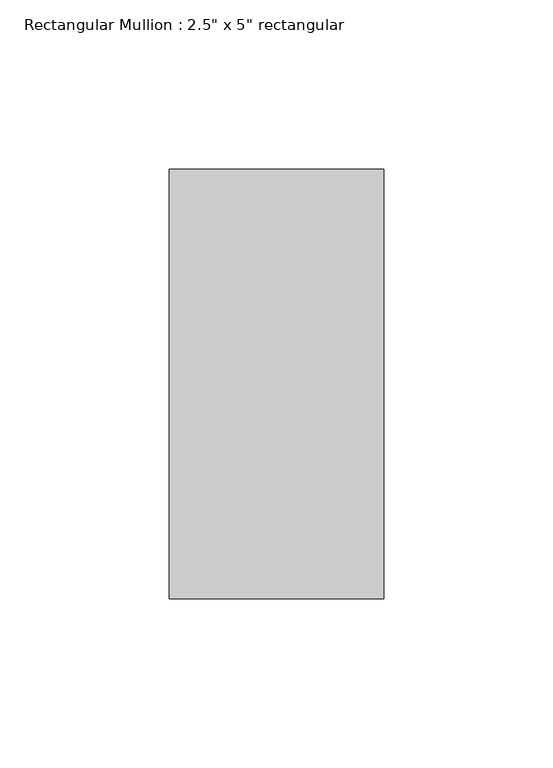
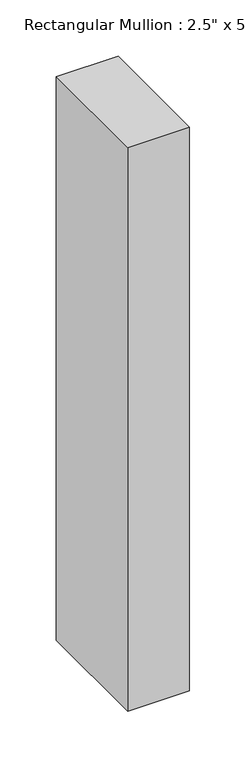
"""IFC4 building model written with IfcOpenShell, lengths in millimetres: member geometry."""

from ifc_helpers import new_model, si_unit, frame, origin, place, context, project, spatial, polyline, outline, extrude, source, transform, mapped, element, save


def member_0fdf3d9d(model_context):
    return source(origin(), model_context, "Body", "SweptSolid", [
        extrude(outline(polyline([(0.0, 63.5), (0.0, -63.5), (-63.5, -63.5), (-63.5, 63.5), (0.0, 63.5)])), frame((0.0, 0.0, -612.775), z_axis=(0.0, 0.0, 1.0), x_axis=(1.0, 0.0, 0.0)), (0.0, 0.0, 1.0), 612.775),
    ])


if __name__ == "__main__":
    model = new_model("IFC4")
    model_context = context("Model", 3, world=origin())
    ifc_project = project(units=[si_unit("LENGTHUNIT", "METRE", prefix="MILLI")], contexts=[model_context])
    site = spatial("IfcSite", under=ifc_project)
    building = spatial("IfcBuilding", under=site)
    placement = place(None, origin())
    member_shape = member_0fdf3d9d(model_context)
    element("IfcMember", 1, ObjectType="Rectangular Mullion : 2.5\" x 5\" rectangular", at=placement, inside=building, context=model_context, shape_type="MappedRepresentation", body=[
        mapped(member_shape, transform((0.0, 0.0, 0.0), x_axis=(1.0, 0.0, 0.0), y_axis=(0.0, 1.0, 0.0), z_axis=(0.0, 0.0, 1.0))),
    ])
    save(model, "model.ifc")

# Revit data of these elements
# Type "Rectangular Mullion : 2.5\" x 5\" rectangular"
#   built-in parameter 1007304 = 0.416667 (stored number, unit not read)
#   built-in parameter 1007301 = 0.104167 (stored number, unit not read)
#   built-in parameter 1007300 = 0.104167 (stored number, unit not read)
# Element 1 (IfcMember, "Rectangular Mullion : 2.5\" x 5\" rectangular")
#   Materials on its faces: "Aluminum"
# Materials
#   "Aluminum": class "Metal", colour RGB 247 247 247, transparency 0, Description = "Aluminum 6061", Cost = 0
